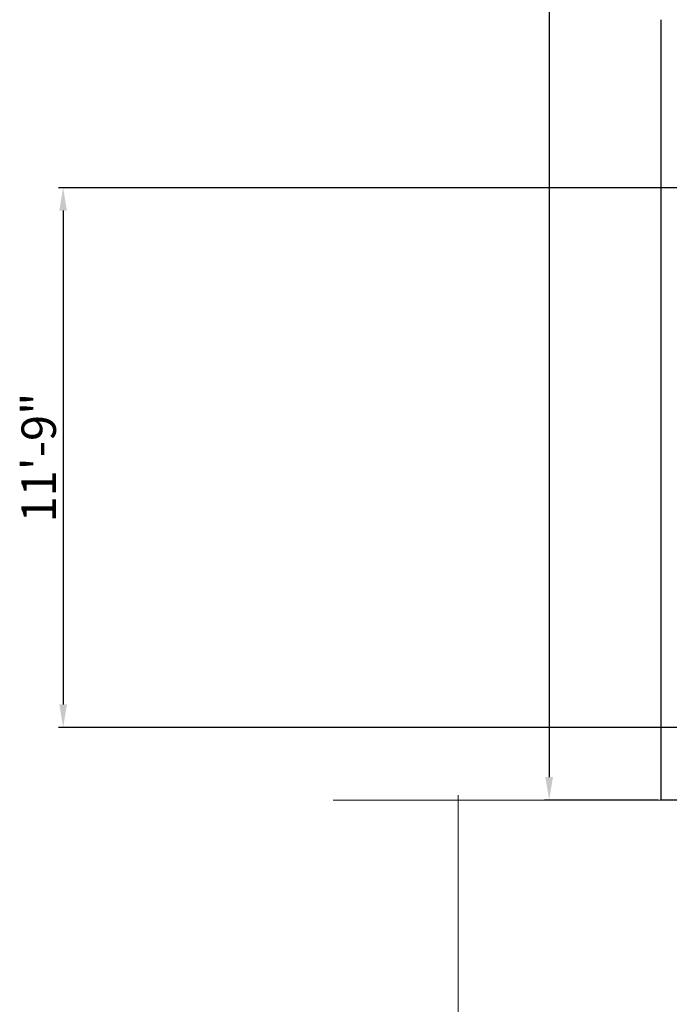
# Model space of a CAD drawing. Units: millimetres. Extents: x 595116 to 630915, y 909473 to 920225.
# Tile 3 of 134: x 629144 to 629314, y 919089 to 919346. Entities that reach past the tile are written whole.
import ezdxf

# ---------------------------------------------------------------- set-up
doc = ezdxf.new("R2010")
doc.units = ezdxf.units.MM
for name, color, linetype, lineweight in [('C-PROP', 7, 'Continuous', 25), ('C-ROAD', 30, 'Continuous', 18), ('Dimension', 3, 'Continuous', 18)]:
    doc.layers.add(name, color=color, linetype=linetype, lineweight=lineweight)
doc.styles.get("Standard").update_dxf_attribs({"font": 'arial.ttf'})
doc.dimstyles.new('ISO-25', dxfattribs={"dimtxt": 9, "dimasz": 6, "dimexe": 1.25, "dimexo": 0.625, "dimtad": 1, "dimlunit": 4, "dimtxsty": 'Standard', "dimcen": 2.5, "dimadec": 0, "dimazin": 0, "dimtfac": 1, "dimtmove": 0, "dimatfit": 3, "dimfxl": 1, "dimarcsym": 0})

# ---------------------------------------------------------------- blocks, each defined once
blk = doc.blocks.new('*D128')
at = {"layer": 'Defpoints', "color": 0, "transparency": 16777216}
for p in [(629311.54, 920089.43), (629282.4, 919141.93), (629311.54, 919141.93)]:
    blk.add_point(p, dxfattribs=at)
at = {"layer": 'Dimension', "color": 0, "lineweight": -2, "transparency": 16777216}
for p, q in [((629310.92, 920089.43), (629281.15, 920089.43)), ((629282.4, 920083.43), (629282.4, 919147.93)), ((629310.92, 919141.93), (629281.15, 919141.93))]:
    blk.add_line(p, q, dxfattribs=at)
at = {"layer": 'Dimension', "color": 0, "transparency": 16777216}
for points in [[(629281.4, 920083.43), (629283.4, 920083.43), (629282.4, 920089.43)], [(629281.4, 919147.93), (629283.4, 919147.93), (629282.4, 919141.93)]]:
    blk.add_solid(points, dxfattribs=at)
at = {"layer": 'Dimension', "color": 0, "transparency": 16777216, "insert": (629271.16, 919615.68), "char_height": 9, "attachment_point": 5, "rotation": 90}
blk.add_mtext('78\'-11{\\H1x;\\S1/2;}"', dxfattribs=at)
blk = doc.blocks.new('*D221')
at = {"layer": 'Defpoints', "color": 0, "transparency": 16777216}
for p in [(629511.27, 919302.01), (629155.38, 919160.92), (629511.27, 919160.92)]:
    blk.add_point(p, dxfattribs=at)
at = {"layer": 'Dimension', "color": 0, "lineweight": -2, "transparency": 16777216}
for p, q in [((629510.65, 919302.01), (629154.13, 919302.01)), ((629155.38, 919296.01), (629155.38, 919166.92)), ((629510.65, 919160.92), (629154.13, 919160.92))]:
    blk.add_line(p, q, dxfattribs=at)
at = {"layer": 'Dimension', "color": 0, "transparency": 16777216}
for points in [[(629154.38, 919296.01), (629156.38, 919296.01), (629155.38, 919302.01)], [(629154.38, 919166.92), (629156.38, 919166.92), (629155.38, 919160.92)]]:
    blk.add_solid(points, dxfattribs=at)
at = {"layer": 'Dimension', "color": 0, "transparency": 16777216, "insert": (629150.16, 919231.46), "char_height": 9, "attachment_point": 5, "rotation": 90}
blk.add_mtext('11\'-9"', dxfattribs=at)

msp = doc.modelspace()

# ---------------------------------------------------------------- linework, layer by layer
at = {"layer": 'C-PROP'}
msp.add_line((629311.541, 919345.928), (629311.541, 919141.928), dxfattribs=at)
msp.add_lwpolyline([(629334.041, 919141.928), (629311.541, 919141.928)], dxfattribs=at)
at = {"layer": 'C-ROAD'}
msp.add_line((629311.541, 919141.928), (629225.95, 919141.928), dxfattribs=at)
msp.add_lwpolyline([(629258.594, 919143.178), (629258.594, 919062.342), (629223.682, 919021.992), (629300.343, 919021.872), (629258.594, 918997.995), (629258.594, 918900.678)], dxfattribs=at)

# ---------------------------------------------------------------- dimensions: what is measured, and where the dimension line sits
at = {"layer": 'Dimension'}
for base, p1, p2, override, picture, middle in [((629282.395, 919141.928), (629311.541, 920089.428), (629311.541, 919141.928), {"dimclrd": 0, "dimclre": 0, "dimclrt": 0}, '*D128', (629271.157, 919615.678)), ((629155.382, 919160.917), (629511.274, 919302.009), (629511.274, 919160.917), {"dimdec": 1, "dimlfac": 1, "dimrnd": 0, "dimzin": 1, "dimdsep": 46, "dimlunit": 4, "dimfrac": 2}, '*D221', (629150.162, 919231.463))]:
    dim = msp.add_linear_dim(base=base, p1=p1, p2=p2, angle=90, dimstyle='ISO-25', override=override, dxfattribs=at)
    dim.commit()
    dim.dimension.update_dxf_attribs({"geometry": picture, "text_midpoint": middle})

doc.saveas('drawing.dxf')
